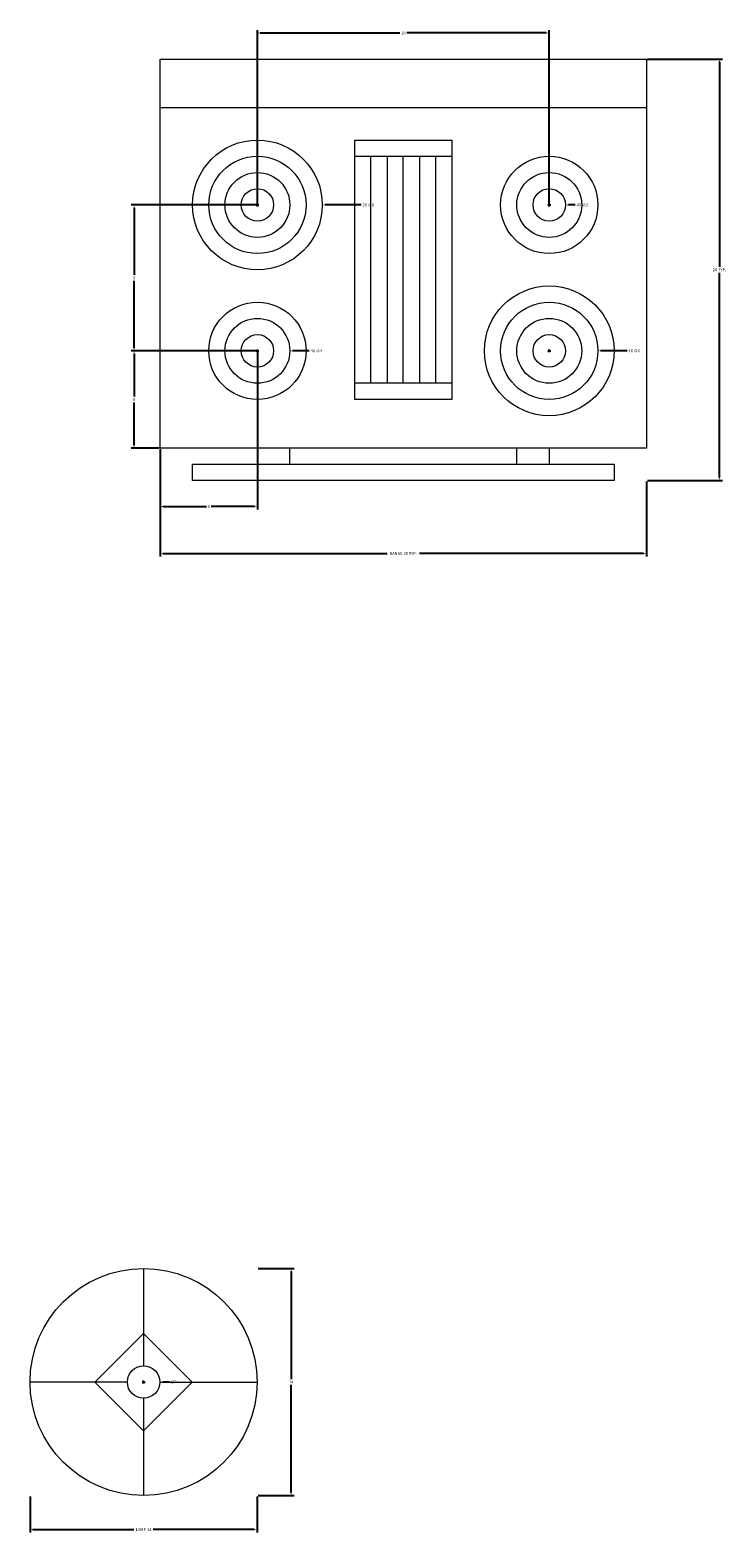
# Model space of a CAD drawing. Units: inches. Extents: x -494 to 1275, y 12 to 1194.
# Tile 7 of 8: x 1080 to 1122, y 824 to 917. Entities that reach past the tile are written whole.
import ezdxf

# ---------------------------------------------------------------- set-up
doc = ezdxf.new("R2010")
doc.units = ezdxf.units.IN
doc.header["$MEASUREMENT"] = 0
for name, color, linetype, lineweight in [('A-ANNO-DIMS', 2, 'Continuous', 18), ('A-EQPM', 8, 'Continuous', 18), ('E-LITE', 8, 'Continuous', 18)]:
    doc.layers.add(name, color=color, linetype=linetype, lineweight=lineweight)
doc.styles.get("Standard").update_dxf_attribs({"font": 'arial.ttf'})
doc.dimstyles.get("Standard").update_dxf_attribs({"dimtxt": 0.18, "dimasz": 0.18, "dimexe": 0.18, "dimexo": 0.0625, "dimgap": 0.09, "dimtad": 0, "dimtih": 1, "dimtoh": 1, "dimdec": 4, "dimzin": 0, "dimdsep": 46, "dimlunit": 4, "dimtxsty": 'Standard', "dimcen": 0.09, "dimadec": 0, "dimazin": 0, "dimtfac": 1, "dimtdec": 4, "dimtofl": 0, "dimtmove": 0, "dimatfit": 3, "dimfxl": 1, "dimtolj": 1, "dimtzin": 0, "dimarcsym": 0})

# ---------------------------------------------------------------- blocks, each defined once
blk = doc.blocks.new('Range-Oven - 30 in top')
for p, q in [((0, -3), (30, -3)), ((12, -6), (18, -6)), ((13, -20), (13, -6)), ((14, -6), (14, -20)), ((15, -20), (15, -6)), ((16, -6), (16, -20)), ((17, -20), (17, -6)), ((18, -20), (12, -20)), ((6, -24), (6, -25)), ((8, -25), (8, -24)), ((22, -25), (22, -24)), ((24, -24), (24, -25))]:
    blk.add_line(p, q)
for points in [[(0, -24), (0, 0), (30, 0), (30, -24)], [(12, -21), (12, -5), (18, -5), (18, -21)], [(2, -26), (2, -25), (28, -25), (28, -26)]]:
    blk.add_lwpolyline(points, close=True)
for centre, radius in [((6, -9), 4), ((6, -9), 3), ((24, -9), 3), ((6, -9), 2), ((24, -9), 2), ((6, -9), 1), ((24, -9), 1), ((24, -18), 4), ((6, -18), 3), ((24, -18), 3), ((6, -18), 2), ((24, -18), 2), ((6, -18), 1), ((24, -18), 1)]:
    blk.add_circle(centre, radius)
blk = doc.blocks.new('Lamp - Table')
for p, q in [((0, 7), (0, 1)), ((0, 3), (-3, 0)), ((3, 0), (0, 3)), ((-1, 0), (-7, 0)), ((-3, 0), (0, -3)), ((0, -3), (3, 0)), ((1, 0), (7, 0)), ((0, -1), (0, -7))]:
    blk.add_line(p, q)
for radius in [7, 1]:
    blk.add_circle((0, 0), radius)
blk = doc.blocks.new('*D26')
at = {"layer": 'A-ANNO-DIMS', "color": 0, "lineweight": -2, "transparency": 16777216}
for p, q in [((1087.536, 888.77), (1087.536, 884.153)), ((1117.536, 888.77), (1117.536, 884.153)), ((1087.716, 884.333), (1101.531, 884.333)), ((1117.356, 884.333), (1103.542, 884.333))]:
    blk.add_line(p, q, dxfattribs=at)
at = {"layer": 'A-ANNO-DIMS', "color": 0, "transparency": 16777216}
for points in [[(1087.716, 884.363), (1087.716, 884.303), (1087.536, 884.333)], [(1117.356, 884.363), (1117.356, 884.303), (1117.536, 884.333)]]:
    blk.add_solid(points, dxfattribs=at)
at = {"layer": 'Defpoints', "color": 0, "transparency": 16777216}
for p in [(1087.536, 888.833), (1117.536, 888.833), (1117.536, 884.333)]:
    blk.add_point(p, dxfattribs=at)
at = {"layer": 'A-ANNO-DIMS', "color": 0, "transparency": 16777216, "insert": (1102.536, 884.333), "char_height": 0.18, "attachment_point": 5}
blk.add_mtext('\\A1;RANGE 30 TYP.', dxfattribs=at)
blk = doc.blocks.new('*D27')
at = {"layer": 'A-ANNO-DIMS', "color": 0, "lineweight": -2, "transparency": 16777216}
for p, q in [((1117.599, 914.833), (1122.216, 914.833)), ((1122.036, 914.653), (1122.036, 902.014)), ((1122.036, 889.013), (1122.036, 901.651)), ((1117.599, 888.833), (1122.216, 888.833))]:
    blk.add_line(p, q, dxfattribs=at)
at = {"layer": 'A-ANNO-DIMS', "color": 0, "transparency": 16777216}
for points in [[(1122.006, 914.653), (1122.066, 914.653), (1122.036, 914.833)], [(1122.006, 889.013), (1122.066, 889.013), (1122.036, 888.833)]]:
    blk.add_solid(points, dxfattribs=at)
at = {"layer": 'Defpoints', "color": 0, "transparency": 16777216}
for p in [(1117.536, 914.833), (1122.036, 914.833), (1117.536, 888.833)]:
    blk.add_point(p, dxfattribs=at)
at = {"layer": 'A-ANNO-DIMS', "color": 0, "transparency": 16777216, "insert": (1122.036, 901.833), "char_height": 0.18, "attachment_point": 5}
blk.add_mtext('\\A1;26 TYP.', dxfattribs=at)
blk = doc.blocks.new('*D38')
at = {"layer": 'A-ANNO-DIMS', "color": 0, "lineweight": -2, "transparency": 16777216}
for p, q in [((1079.515, 826.165), (1079.515, 823.948)), ((1093.515, 826.165), (1093.515, 823.948)), ((1079.695, 824.128), (1085.923, 824.128)), ((1093.335, 824.128), (1087.107, 824.128))]:
    blk.add_line(p, q, dxfattribs=at)
at = {"layer": 'A-ANNO-DIMS', "color": 0, "transparency": 16777216}
for points in [[(1079.695, 824.158), (1079.695, 824.098), (1079.515, 824.128)], [(1093.335, 824.158), (1093.335, 824.098), (1093.515, 824.128)]]:
    blk.add_solid(points, dxfattribs=at)
at = {"layer": 'Defpoints', "color": 0, "transparency": 16777216}
for p in [(1079.515, 826.228), (1093.515, 826.228), (1093.515, 824.128)]:
    blk.add_point(p, dxfattribs=at)
at = {"layer": 'A-ANNO-DIMS', "color": 0, "transparency": 16777216, "insert": (1086.515, 824.128), "char_height": 0.18, "attachment_point": 5}
blk.add_mtext('\\A1;LAMP 14', dxfattribs=at)
blk = doc.blocks.new('*D39')
at = {"layer": 'A-ANNO-DIMS', "color": 0, "lineweight": -2, "transparency": 16777216}
for p, q in [((1093.578, 840.228), (1095.795, 840.228)), ((1095.615, 840.048), (1095.615, 833.408)), ((1095.615, 826.408), (1095.615, 833.047)), ((1093.578, 826.228), (1095.795, 826.228))]:
    blk.add_line(p, q, dxfattribs=at)
at = {"layer": 'A-ANNO-DIMS', "color": 0, "transparency": 16777216}
for points in [[(1095.585, 840.048), (1095.645, 840.048), (1095.615, 840.228)], [(1095.585, 826.408), (1095.645, 826.408), (1095.615, 826.228)]]:
    blk.add_solid(points, dxfattribs=at)
at = {"layer": 'Defpoints', "color": 0, "transparency": 16777216}
for p in [(1093.515, 840.228), (1095.615, 840.228), (1093.515, 826.228)]:
    blk.add_point(p, dxfattribs=at)
at = {"layer": 'A-ANNO-DIMS', "color": 0, "transparency": 16777216, "insert": (1095.615, 833.228), "char_height": 0.18, "attachment_point": 5}
blk.add_mtext('\\A1;14', dxfattribs=at)
blk = doc.blocks.new('*D73')
at = {"layer": 'A-ANNO-DIMS', "color": 0, "lineweight": -2, "transparency": 16777216}
for p, q in [((1093.536, 905.895), (1093.536, 916.618)), ((1111.536, 905.895), (1111.536, 916.618)), ((1093.716, 916.438), (1102.325, 916.438)), ((1111.356, 916.438), (1102.747, 916.438))]:
    blk.add_line(p, q, dxfattribs=at)
at = {"layer": 'A-ANNO-DIMS', "color": 0, "transparency": 16777216}
for points in [[(1093.716, 916.468), (1093.716, 916.408), (1093.536, 916.438)], [(1111.356, 916.468), (1111.356, 916.408), (1111.536, 916.438)]]:
    blk.add_solid(points, dxfattribs=at)
at = {"layer": 'Defpoints', "color": 0, "transparency": 16777216}
for p in [(1111.536, 916.438), (1093.536, 905.833), (1111.536, 905.833)]:
    blk.add_point(p, dxfattribs=at)
at = {"layer": 'A-ANNO-DIMS', "color": 0, "transparency": 16777216, "insert": (1102.536, 916.438), "char_height": 0.18, "attachment_point": 5}
blk.add_mtext('\\A1;18', dxfattribs=at)
blk = doc.blocks.new('*D74')
at = {"layer": 'A-ANNO-DIMS', "color": 0, "lineweight": -2, "transparency": 16777216}
for p, q in [((1093.474, 905.833), (1085.751, 905.833)), ((1085.931, 905.653), (1085.931, 901.514)), ((1085.931, 897.013), (1085.931, 901.151)), ((1093.474, 896.833), (1085.751, 896.833))]:
    blk.add_line(p, q, dxfattribs=at)
at = {"layer": 'A-ANNO-DIMS', "color": 0, "transparency": 16777216}
for points in [[(1085.901, 905.653), (1085.961, 905.653), (1085.931, 905.833)], [(1085.901, 897.013), (1085.961, 897.013), (1085.931, 896.833)]]:
    blk.add_solid(points, dxfattribs=at)
at = {"layer": 'Defpoints', "color": 0, "transparency": 16777216}
for p in [(1085.931, 905.833), (1093.536, 905.833), (1093.536, 896.833)]:
    blk.add_point(p, dxfattribs=at)
at = {"layer": 'A-ANNO-DIMS', "color": 0, "transparency": 16777216, "insert": (1085.931, 901.333), "char_height": 0.18, "attachment_point": 5}
blk.add_mtext('\\A1;9', dxfattribs=at)
blk = doc.blocks.new('*D91')
at = {"layer": 'A-ANNO-DIMS', "color": 0, "lineweight": -2, "transparency": 16777216}
for p, q in [((1093.536, 896.77), (1093.536, 887.048)), ((1087.536, 890.77), (1087.536, 887.048)), ((1087.716, 887.228), (1090.387, 887.228)), ((1093.356, 887.228), (1090.686, 887.228))]:
    blk.add_line(p, q, dxfattribs=at)
at = {"layer": 'A-ANNO-DIMS', "color": 0, "transparency": 16777216}
for points in [[(1087.716, 887.258), (1087.716, 887.198), (1087.536, 887.228)], [(1093.356, 887.258), (1093.356, 887.198), (1093.536, 887.228)]]:
    blk.add_solid(points, dxfattribs=at)
at = {"layer": 'Defpoints', "color": 0, "transparency": 16777216}
for p in [(1093.536, 896.833), (1087.536, 890.833), (1087.536, 887.228)]:
    blk.add_point(p, dxfattribs=at)
at = {"layer": 'A-ANNO-DIMS', "color": 0, "transparency": 16777216, "insert": (1090.536, 887.228), "char_height": 0.18, "attachment_point": 5}
blk.add_mtext('\\A1;6', dxfattribs=at)
blk = doc.blocks.new('*D92')
at = {"layer": 'A-ANNO-DIMS', "color": 0, "lineweight": -2, "transparency": 16777216}
for p, q in [((1093.474, 896.833), (1085.751, 896.833)), ((1085.931, 896.653), (1085.931, 894.014)), ((1085.931, 891.013), (1085.931, 893.651)), ((1087.474, 890.833), (1085.751, 890.833))]:
    blk.add_line(p, q, dxfattribs=at)
at = {"layer": 'A-ANNO-DIMS', "color": 0, "transparency": 16777216}
for points in [[(1085.901, 896.653), (1085.961, 896.653), (1085.931, 896.833)], [(1085.901, 891.013), (1085.961, 891.013), (1085.931, 890.833)]]:
    blk.add_solid(points, dxfattribs=at)
at = {"layer": 'Defpoints', "color": 0, "transparency": 16777216}
for p in [(1093.536, 896.833), (1085.931, 890.833), (1087.536, 890.833)]:
    blk.add_point(p, dxfattribs=at)
at = {"layer": 'A-ANNO-DIMS', "color": 0, "transparency": 16777216, "insert": (1085.931, 893.833), "char_height": 0.18, "attachment_point": 5}
blk.add_mtext('\\A1;6', dxfattribs=at)
blk = doc.blocks.new('*D100')
at = {"layer": 'A-ANNO-DIMS', "color": 0, "lineweight": -2, "transparency": 16777216}
for p, q in [((1086.425, 833.228), (1086.605, 833.228)), ((1086.515, 833.138), (1086.515, 833.318)), ((1088.115, 833.228), (1087.695, 833.228))]:
    blk.add_line(p, q, dxfattribs=at)
at = {"layer": 'A-ANNO-DIMS', "color": 0, "transparency": 16777216}
blk.add_solid([(1087.695, 833.258), (1087.695, 833.198), (1087.515, 833.228)], dxfattribs=at)
at = {"layer": 'Defpoints', "color": 0, "transparency": 16777216}
for p in [(1085.515, 833.228), (1087.515, 833.228)]:
    blk.add_point(p, dxfattribs=at)
at = {"layer": 'A-ANNO-DIMS', "color": 0, "transparency": 16777216, "insert": (1088.361, 833.228), "char_height": 0.18, "attachment_point": 5}
blk.add_mtext('\\A1;∅2', dxfattribs=at)
blk = doc.blocks.new('*D101')
at = {"layer": 'A-ANNO-DIMS', "color": 0, "lineweight": -2, "transparency": 16777216}
for p, q in [((1093.446, 905.833), (1093.626, 905.833)), ((1093.536, 905.743), (1093.536, 905.923)), ((1099.936, 905.833), (1097.716, 905.833))]:
    blk.add_line(p, q, dxfattribs=at)
at = {"layer": 'A-ANNO-DIMS', "color": 0, "transparency": 16777216}
blk.add_solid([(1097.716, 905.863), (1097.716, 905.803), (1097.536, 905.833)], dxfattribs=at)
at = {"layer": 'Defpoints', "color": 0, "transparency": 16777216}
for p in [(1089.536, 905.832), (1097.536, 905.833)]:
    blk.add_point(p, dxfattribs=at)
at = {"layer": 'A-ANNO-DIMS', "color": 0, "transparency": 16777216, "insert": (1100.373, 905.833), "char_height": 0.18, "attachment_point": 5}
blk.add_mtext('\\A1;2X ∅8', dxfattribs=at)
blk = doc.blocks.new('*D102')
at = {"layer": 'A-ANNO-DIMS', "color": 0, "lineweight": -2, "transparency": 16777216}
for p, q in [((1111.446, 896.833), (1111.626, 896.833)), ((1111.536, 896.743), (1111.536, 896.923)), ((1116.336, 896.833), (1114.716, 896.833))]:
    blk.add_line(p, q, dxfattribs=at)
at = {"layer": 'A-ANNO-DIMS', "color": 0, "transparency": 16777216}
blk.add_solid([(1114.716, 896.863), (1114.716, 896.803), (1114.536, 896.833)], dxfattribs=at)
at = {"layer": 'Defpoints', "color": 0, "transparency": 16777216}
for p in [(1108.536, 896.832), (1114.536, 896.833)]:
    blk.add_point(p, dxfattribs=at)
at = {"layer": 'A-ANNO-DIMS', "color": 0, "transparency": 16777216, "insert": (1116.775, 896.833), "char_height": 0.18, "attachment_point": 5}
blk.add_mtext('\\A1;4X ∅6', dxfattribs=at)
blk = doc.blocks.new('*D103')
at = {"layer": 'A-ANNO-DIMS', "color": 0, "lineweight": -2, "transparency": 16777216}
for p, q in [((1093.446, 896.833), (1093.626, 896.833)), ((1093.536, 896.743), (1093.536, 896.923)), ((1096.736, 896.833), (1095.716, 896.833))]:
    blk.add_line(p, q, dxfattribs=at)
at = {"layer": 'A-ANNO-DIMS', "color": 0, "transparency": 16777216}
blk.add_solid([(1095.716, 896.863), (1095.716, 896.803), (1095.536, 896.833)], dxfattribs=at)
at = {"layer": 'Defpoints', "color": 0, "transparency": 16777216}
for p in [(1091.536, 896.832), (1095.536, 896.833)]:
    blk.add_point(p, dxfattribs=at)
at = {"layer": 'A-ANNO-DIMS', "color": 0, "transparency": 16777216, "insert": (1097.175, 896.833), "char_height": 0.18, "attachment_point": 5}
blk.add_mtext('\\A1;4X ∅4', dxfattribs=at)
blk = doc.blocks.new('*D104')
at = {"layer": 'A-ANNO-DIMS', "color": 0, "lineweight": -2, "transparency": 16777216}
for p, q in [((1111.446, 905.833), (1111.626, 905.833)), ((1111.536, 905.743), (1111.536, 905.923)), ((1113.136, 905.833), (1112.716, 905.833))]:
    blk.add_line(p, q, dxfattribs=at)
at = {"layer": 'A-ANNO-DIMS', "color": 0, "transparency": 16777216}
blk.add_solid([(1112.716, 905.863), (1112.716, 905.803), (1112.536, 905.833)], dxfattribs=at)
at = {"layer": 'Defpoints', "color": 0, "transparency": 16777216}
for p in [(1110.536, 905.832), (1112.536, 905.833)]:
    blk.add_point(p, dxfattribs=at)
at = {"layer": 'A-ANNO-DIMS', "color": 0, "transparency": 16777216, "insert": (1113.574, 905.833), "char_height": 0.18, "attachment_point": 5}
blk.add_mtext('\\A1;4X ∅2', dxfattribs=at)

msp = doc.modelspace()

# ---------------------------------------------------------------- block references
at = {"layer": 'A-EQPM'}
msp.add_blockref('Range-Oven - 30 in top', (1087.5361, 914.8325), dxfattribs=at)
at = {"layer": 'E-LITE'}
msp.add_blockref('Lamp - Table', (1086.5153, 833.2278), dxfattribs=at)

# ---------------------------------------------------------------- dimensions: what is measured, and where the dimension line sits
at = {"layer": 'A-ANNO-DIMS'}
for base, p1, p2, picture, middle in [((1111.5361, 916.4375), (1093.5361, 905.8325), (1111.5361, 905.8325), '*D73', (1102.5361, 916.4375)), ((1087.5361, 887.2275), (1093.5361, 896.8325), (1087.5361, 890.8325), '*D91', (1090.5361, 887.2275))]:
    dim = msp.add_linear_dim(base=base, p1=p1, p2=p2, dimstyle='Standard', override={"dimdec": 0, "dimlfac": 1, "dimrnd": 0, "dimzin": 0, "dimdsep": 46, "dimlunit": 2}, dxfattribs=at)
    dim.commit()
    dim.dimension.update_dxf_attribs({"geometry": picture, "text_midpoint": middle})
dim = msp.add_linear_dim(base=(1122.0361, 914.8325), p1=(1117.5361, 888.8325), p2=(1117.5361, 914.8325), angle=90, text='<> TYP.', dimstyle='Standard', override={"dimdec": 0, "dimlfac": 1, "dimrnd": 0, "dimzin": 0, "dimdsep": 46, "dimlunit": 2}, dxfattribs=at)
dim.commit()
dim.dimension.update_dxf_attribs({"geometry": '*D27', "text_midpoint": (1122.0361, 901.8325)})
for base, p1, p2, picture, middle in [((1085.9311, 905.8325), (1093.5361, 896.8325), (1093.5361, 905.8325), '*D74', (1085.9311, 901.3325)), ((1085.9311, 890.8325), (1093.5361, 896.8325), (1087.5361, 890.8325), '*D92', (1085.9311, 893.8325)), ((1095.6153, 840.2278), (1093.5153, 826.2278), (1093.5153, 840.2278), '*D39', (1095.6153, 833.2278))]:
    dim = msp.add_linear_dim(base=base, p1=p1, p2=p2, angle=90, dimstyle='Standard', override={"dimdec": 0, "dimlfac": 1, "dimrnd": 0, "dimzin": 0, "dimdsep": 46, "dimlunit": 2}, dxfattribs=at)
    dim.commit()
    dim.dimension.update_dxf_attribs({"geometry": picture, "text_midpoint": middle})
for p1, p2, text, picture, middle in [((1089.5361, 905.8321), (1097.5361, 905.833), '2X <>', '*D101', (1099.9361, 905.8333)), ((1110.5361, 905.8321), (1112.5361, 905.833), '4X <>', '*D104', (1113.1361, 905.8333)), ((1091.5361, 896.8321), (1095.5361, 896.833), '4X <>', '*D103', (1096.7361, 896.8333)), ((1108.5361, 896.8321), (1114.5361, 896.833), '4X <>', '*D102', (1116.3361, 896.8333))]:
    dim = msp.add_diameter_dim_2p(p1=p1, p2=p2, text=text, dimstyle='Standard', override={"dimdec": 0, "dimlfac": 1, "dimrnd": 0, "dimzin": 0, "dimdsep": 46, "dimlunit": 2}, dxfattribs=at)
    dim.commit()
    dim.dimension.update_dxf_attribs({"geometry": picture, "text_midpoint": middle, "dimtype": 163})
for base, p1, p2, text, picture, middle in [((1117.5361, 884.3325), (1087.5361, 888.8325), (1117.5361, 888.8325), 'RANGE <> TYP.', '*D26', (1102.5361, 884.3325)), ((1093.5153, 824.1278), (1079.5153, 826.2278), (1093.5153, 826.2278), 'LAMP <>', '*D38', (1086.5153, 824.1278))]:
    dim = msp.add_linear_dim(base=base, p1=p1, p2=p2, text=text, dimstyle='Standard', override={"dimdec": 0, "dimlfac": 1, "dimrnd": 0, "dimzin": 0, "dimdsep": 46, "dimlunit": 2}, dxfattribs=at)
    dim.commit()
    dim.dimension.update_dxf_attribs({"geometry": picture, "text_midpoint": middle})
dim = msp.add_diameter_dim_2p(p1=(1085.5153, 833.2275), p2=(1087.5153, 833.228), dimstyle='Standard', override={"dimdec": 0, "dimlfac": 1, "dimrnd": 0, "dimzin": 0, "dimdsep": 46, "dimlunit": 2}, dxfattribs=at)
dim.commit()
dim.dimension.update_dxf_attribs({"geometry": '*D100', "text_midpoint": (1088.1153, 833.2281), "dimtype": 163})

doc.saveas('drawing.dxf')
